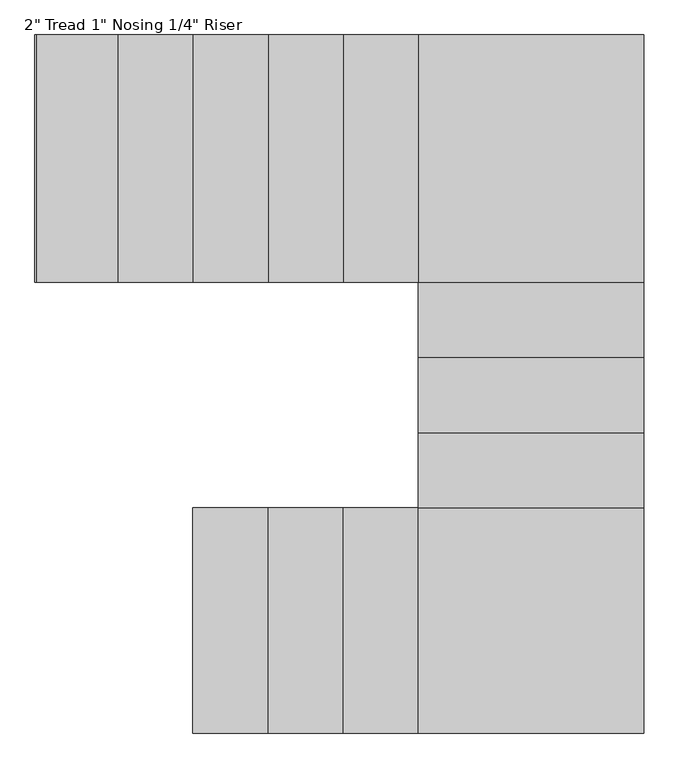
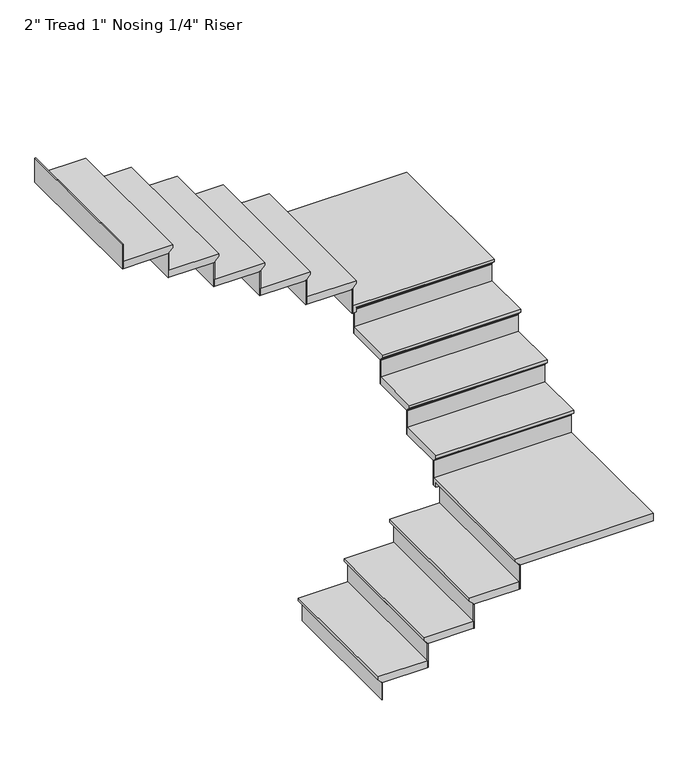
"""IFC4 building model written with IfcOpenShell, lengths in millimetres: stair flight geometry."""

from ifc_helpers import new_model, si_unit, origin, place, context, project, spatial, faceted_brep, source, transform, mapped, element, save


def stair_flight_68b2e5de(model_context):
    return source(origin(), model_context, "Body", "Brep", [
        faceted_brep([(938.5174794, -182.0870507, 16152.2833333), (938.5174794, -182.0870507, 16171.3333333), (938.5174794, 732.3129493, 16171.3333333), (938.5174794, 732.3129493, 16152.2833333), (963.9174794, -182.0870507, 16126.8833333), (963.9174794, 732.3129493, 16126.8833333), (1268.7174794, -182.0870507, 16171.3333333), (1268.7174794, 732.3129493, 16171.3333333), (963.9174794, 732.3129493, 16120.5333333), (1268.7174794, 732.3129493, 16120.5333333), (1268.7174794, -182.0870507, 16120.5333333), (963.9174794, -182.0870507, 16120.5333333)], [[[0, 1, 2, 3]], [[4, 0, 3, 5]], [[2, 1, 6, 7]], [[8, 9, 10, 11]], [[2, 7, 9, 8, 5, 3]], [[8, 11, 4, 5]], [[6, 1, 0, 4, 11, 10]], [[7, 6, 10, 9]]]),
        faceted_brep([(963.9174794, -182.0870507, 16120.5333333), (963.9174794, -182.0870507, 16002.0), (970.2674794, -182.0870507, 16002.0), (970.2674794, -182.0870507, 16120.5333333), (963.9174794, 732.3129493, 16120.5333333), (970.2674794, 732.3129493, 16120.5333333), (970.2674794, 732.3129493, 16002.0), (963.9174794, 732.3129493, 16002.0)], [[[0, 1, 2, 3]], [[4, 5, 6, 7]], [[1, 0, 4, 7]], [[2, 1, 7, 6]], [[3, 2, 6, 5]], [[0, 3, 5, 4]]]),
        faceted_brep([(1268.7174794, -182.0870507, 16289.8666667), (1268.7174794, -182.0870507, 16120.5333333), (1275.0674794, -182.0870507, 16120.5333333), (1275.0674794, -182.0870507, 16289.8666667), (1268.7174794, 732.3129493, 16289.8666667), (1275.0674794, 732.3129493, 16289.8666667), (1275.0674794, 732.3129493, 16120.5333333), (1268.7174794, 732.3129493, 16120.5333333)], [[[0, 1, 2, 3]], [[4, 5, 6, 7]], [[1, 0, 4, 7]], [[2, 1, 7, 6]], [[3, 2, 6, 5]], [[0, 3, 5, 4]]]),
        faceted_brep([(1243.3174794, 732.3129493, 16340.6666667), (1243.3174794, -182.0870507, 16340.6666667), (1573.5174794, -182.0870507, 16340.6666667), (1573.5174794, 732.3129493, 16340.6666667), (1268.7174794, 732.3129493, 16289.8666667), (1573.5174794, 732.3129493, 16289.8666667), (1573.5174794, -182.0870507, 16289.8666667), (1268.7174794, -182.0870507, 16289.8666667), (1268.7174794, 732.3129493, 16296.2166667), (1243.3174794, 732.3129493, 16321.6166667), (1268.7174794, -182.0870507, 16296.2166667), (1243.3174794, -182.0870507, 16321.6166667)], [[[0, 1, 2, 3]], [[4, 5, 6, 7]], [[0, 3, 5, 4, 8, 9]], [[4, 7, 10, 8]], [[2, 1, 11, 10, 7, 6]], [[3, 2, 6, 5]], [[11, 1, 0, 9]], [[10, 11, 9, 8]]]),
        faceted_brep([(1573.5174794, -182.0870507, 16459.2), (1573.5174794, -182.0870507, 16289.8666667), (1579.8674794, -182.0870507, 16289.8666667), (1579.8674794, -182.0870507, 16459.2), (1573.5174794, 732.3129493, 16459.2), (1579.8674794, 732.3129493, 16459.2), (1579.8674794, 732.3129493, 16289.8666667), (1573.5174794, 732.3129493, 16289.8666667)], [[[0, 1, 2, 3]], [[4, 5, 6, 7]], [[1, 0, 4, 7]], [[2, 1, 7, 6]], [[3, 2, 6, 5]], [[0, 3, 5, 4]]]),
        faceted_brep([(1548.1174794, 732.3129493, 16510.0), (1548.1174794, -182.0870507, 16510.0), (1878.3174794, -182.0870507, 16510.0), (1878.3174794, 732.3129493, 16510.0), (1573.5174794, 732.3129493, 16459.2), (1878.3174794, 732.3129493, 16459.2), (1878.3174794, -182.0870507, 16459.2), (1573.5174794, -182.0870507, 16459.2), (1573.5174794, 732.3129493, 16465.55), (1548.1174794, 732.3129493, 16490.95), (1573.5174794, -182.0870507, 16465.55), (1548.1174794, -182.0870507, 16490.95)], [[[0, 1, 2, 3]], [[4, 5, 6, 7]], [[0, 3, 5, 4, 8, 9]], [[4, 7, 10, 8]], [[2, 1, 11, 10, 7, 6]], [[3, 2, 6, 5]], [[11, 1, 0, 9]], [[10, 11, 9, 8]]]),
        faceted_brep([(1878.3174794, -182.0870507, 16628.5333333), (1878.3174794, -182.0870507, 16459.2), (1884.6674794, -182.0870507, 16459.2), (1884.6674794, -182.0870507, 16628.5333333), (1878.3174794, 732.3129493, 16628.5333333), (1884.6674794, 732.3129493, 16628.5333333), (1884.6674794, 732.3129493, 16459.2), (1878.3174794, 732.3129493, 16459.2)], [[[0, 1, 2, 3]], [[4, 5, 6, 7]], [[1, 0, 4, 7]], [[2, 1, 7, 6]], [[3, 2, 6, 5]], [[0, 3, 5, 4]]]),
        faceted_brep([(2767.3174794, -182.0870507, 16679.3333333), (2767.3174794, 757.7129493, 16679.3333333), (1852.9174794, 757.7129493, 16679.3333333), (1852.9174794, -182.0870507, 16679.3333333), (1852.9174794, 732.3129493, 16628.5333333), (1852.9174794, 757.7129493, 16628.5333333), (2767.3174794, 757.7129493, 16628.5333333), (2767.3174794, -182.0870507, 16628.5333333), (1878.3174794, -182.0870507, 16628.5333333), (1878.3174794, 732.3129493, 16628.5333333), (1852.9174794, 732.3129493, 16660.2833333), (1852.9174794, -182.0870507, 16660.2833333), (1878.3174794, 732.3129493, 16634.8833333), (1878.3174794, -182.0870507, 16634.8833333)], [[[0, 1, 2, 3]], [[4, 5, 6, 7, 8, 9]], [[3, 2, 5, 4, 10, 11]], [[4, 9, 12, 10]], [[9, 8, 13, 12]], [[0, 3, 11, 13, 8, 7]], [[1, 0, 7, 6]], [[2, 1, 6, 5]], [[13, 11, 10, 12]]]),
        faceted_brep([(2767.3174794, 757.7129493, 16797.8666667), (2767.3174794, 757.7129493, 16628.5333333), (2767.3174794, 764.0629493, 16628.5333333), (2767.3174794, 764.0629493, 16797.8666667), (1852.9174794, 757.7129493, 16797.8666667), (1852.9174794, 764.0629493, 16797.8666667), (1852.9174794, 764.0629493, 16628.5333333), (1852.9174794, 757.7129493, 16628.5333333)], [[[0, 1, 2, 3]], [[4, 5, 6, 7]], [[1, 0, 4, 7]], [[2, 1, 7, 6]], [[3, 2, 6, 5]], [[0, 3, 5, 4]]]),
        faceted_brep([(1852.9174794, 732.3129493, 16848.6666667), (2767.3174794, 732.3129493, 16848.6666667), (2767.3174794, 1062.5129493, 16848.6666667), (1852.9174794, 1062.5129493, 16848.6666667), (1852.9174794, 757.7129493, 16797.8666667), (1852.9174794, 1062.5129493, 16797.8666667), (2767.3174794, 1062.5129493, 16797.8666667), (2767.3174794, 757.7129493, 16797.8666667), (1852.9174794, 757.7129493, 16804.2166667), (1852.9174794, 732.3129493, 16829.6166667), (2767.3174794, 757.7129493, 16804.2166667), (2767.3174794, 732.3129493, 16829.6166667)], [[[0, 1, 2, 3]], [[4, 5, 6, 7]], [[0, 3, 5, 4, 8, 9]], [[4, 7, 10, 8]], [[2, 1, 11, 10, 7, 6]], [[3, 2, 6, 5]], [[11, 1, 0, 9]], [[10, 11, 9, 8]]]),
        faceted_brep([(2767.3174794, 1062.5129493, 16967.2), (2767.3174794, 1062.5129493, 16797.8666667), (2767.3174794, 1068.8629493, 16797.8666667), (2767.3174794, 1068.8629493, 16967.2), (1852.9174794, 1062.5129493, 16967.2), (1852.9174794, 1068.8629493, 16967.2), (1852.9174794, 1068.8629493, 16797.8666667), (1852.9174794, 1062.5129493, 16797.8666667)], [[[0, 1, 2, 3]], [[4, 5, 6, 7]], [[1, 0, 4, 7]], [[2, 1, 7, 6]], [[3, 2, 6, 5]], [[0, 3, 5, 4]]]),
        faceted_brep([(1852.9174794, 1037.1129493, 17018.0), (2767.3174794, 1037.1129493, 17018.0), (2767.3174794, 1367.3129493, 17018.0), (1852.9174794, 1367.3129493, 17018.0), (1852.9174794, 1062.5129493, 16967.2), (1852.9174794, 1367.3129493, 16967.2), (2767.3174794, 1367.3129493, 16967.2), (2767.3174794, 1062.5129493, 16967.2), (1852.9174794, 1062.5129493, 16973.55), (1852.9174794, 1037.1129493, 16998.95), (2767.3174794, 1062.5129493, 16973.55), (2767.3174794, 1037.1129493, 16998.95)], [[[0, 1, 2, 3]], [[4, 5, 6, 7]], [[0, 3, 5, 4, 8, 9]], [[4, 7, 10, 8]], [[2, 1, 11, 10, 7, 6]], [[3, 2, 6, 5]], [[11, 1, 0, 9]], [[10, 11, 9, 8]]]),
        faceted_brep([(2767.3174794, 1367.3129493, 17136.5333333), (2767.3174794, 1367.3129493, 16967.2), (2767.3174794, 1373.6629493, 16967.2), (2767.3174794, 1373.6629493, 17136.5333333), (1852.9174794, 1367.3129493, 17136.5333333), (1852.9174794, 1373.6629493, 17136.5333333), (1852.9174794, 1373.6629493, 16967.2), (1852.9174794, 1367.3129493, 16967.2)], [[[0, 1, 2, 3]], [[4, 5, 6, 7]], [[1, 0, 4, 7]], [[2, 1, 7, 6]], [[3, 2, 6, 5]], [[0, 3, 5, 4]]]),
        faceted_brep([(1852.9174794, 1341.9129493, 17187.3333333), (2767.3174794, 1341.9129493, 17187.3333333), (2767.3174794, 1672.1129493, 17187.3333333), (1852.9174794, 1672.1129493, 17187.3333333), (1852.9174794, 1367.3129493, 17136.5333333), (1852.9174794, 1672.1129493, 17136.5333333), (2767.3174794, 1672.1129493, 17136.5333333), (2767.3174794, 1367.3129493, 17136.5333333), (1852.9174794, 1367.3129493, 17142.8833333), (1852.9174794, 1341.9129493, 17168.2833333), (2767.3174794, 1367.3129493, 17142.8833333), (2767.3174794, 1341.9129493, 17168.2833333)], [[[0, 1, 2, 3]], [[4, 5, 6, 7]], [[0, 3, 5, 4, 8, 9]], [[4, 7, 10, 8]], [[2, 1, 11, 10, 7, 6]], [[3, 2, 6, 5]], [[11, 1, 0, 9]], [[10, 11, 9, 8]]]),
        faceted_brep([(2767.3174794, 1672.1129493, 17305.8666667), (2767.3174794, 1672.1129493, 17136.5333333), (2767.3174794, 1678.4629493, 17136.5333333), (2767.3174794, 1678.4629493, 17305.8666667), (1852.9174794, 1672.1129493, 17305.8666667), (1852.9174794, 1678.4629493, 17305.8666667), (1852.9174794, 1678.4629493, 17136.5333333), (1852.9174794, 1672.1129493, 17136.5333333)], [[[0, 1, 2, 3]], [[4, 5, 6, 7]], [[1, 0, 4, 7]], [[2, 1, 7, 6]], [[3, 2, 6, 5]], [[0, 3, 5, 4]]]),
        faceted_brep([(2767.3174794, 2650.0129493, 17356.6666667), (1827.5174794, 2650.0129493, 17356.6666667), (1827.5174794, 1646.7129493, 17356.6666667), (2767.3174794, 1646.7129493, 17356.6666667), (1852.9174794, 1646.7129493, 17305.8666667), (1827.5174794, 1646.7129493, 17305.8666667), (1827.5174794, 2650.0129493, 17305.8666667), (2767.3174794, 2650.0129493, 17305.8666667), (2767.3174794, 1672.1129493, 17305.8666667), (1852.9174794, 1672.1129493, 17305.8666667), (1852.9174794, 1646.7129493, 17337.6166667), (2767.3174794, 1646.7129493, 17337.6166667), (1852.9174794, 1672.1129493, 17312.2166667), (2767.3174794, 1672.1129493, 17312.2166667)], [[[0, 1, 2, 3]], [[4, 5, 6, 7, 8, 9]], [[3, 2, 5, 4, 10, 11]], [[4, 9, 12, 10]], [[9, 8, 13, 12]], [[0, 3, 11, 13, 8, 7]], [[1, 0, 7, 6]], [[2, 1, 6, 5]], [[13, 11, 10, 12]]]),
        faceted_brep([(1827.5174794, 2650.0129493, 17475.2), (1827.5174794, 2650.0129493, 17305.8666667), (1821.1674794, 2650.0129493, 17305.8666667), (1821.1674794, 2650.0129493, 17475.2), (1827.5174794, 1646.7129493, 17475.2), (1821.1674794, 1646.7129493, 17475.2), (1821.1674794, 1646.7129493, 17305.8666667), (1827.5174794, 1646.7129493, 17305.8666667)], [[[0, 1, 2, 3]], [[4, 5, 6, 7]], [[1, 0, 4, 7]], [[2, 1, 7, 6]], [[3, 2, 6, 5]], [[0, 3, 5, 4]]]),
        faceted_brep([(1852.9174794, 1646.7129493, 17526.0), (1852.9174794, 2650.0129493, 17526.0), (1522.7174794, 2650.0129493, 17526.0), (1522.7174794, 1646.7129493, 17526.0), (1827.5174794, 1646.7129493, 17475.2), (1522.7174794, 1646.7129493, 17475.2), (1522.7174794, 2650.0129493, 17475.2), (1827.5174794, 2650.0129493, 17475.2), (1827.5174794, 1646.7129493, 17481.55), (1852.9174794, 1646.7129493, 17506.95), (1827.5174794, 2650.0129493, 17481.55), (1852.9174794, 2650.0129493, 17506.95)], [[[0, 1, 2, 3]], [[4, 5, 6, 7]], [[0, 3, 5, 4, 8, 9]], [[4, 7, 10, 8]], [[2, 1, 11, 10, 7, 6]], [[3, 2, 6, 5]], [[11, 1, 0, 9]], [[10, 11, 9, 8]]]),
        faceted_brep([(1522.7174794, 2650.0129493, 17644.5333333), (1522.7174794, 2650.0129493, 17475.2), (1516.3674794, 2650.0129493, 17475.2), (1516.3674794, 2650.0129493, 17644.5333333), (1522.7174794, 1646.7129493, 17644.5333333), (1516.3674794, 1646.7129493, 17644.5333333), (1516.3674794, 1646.7129493, 17475.2), (1522.7174794, 1646.7129493, 17475.2)], [[[0, 1, 2, 3]], [[4, 5, 6, 7]], [[1, 0, 4, 7]], [[2, 1, 7, 6]], [[3, 2, 6, 5]], [[0, 3, 5, 4]]]),
        faceted_brep([(1548.1174794, 1646.7129493, 17695.3333333), (1548.1174794, 2650.0129493, 17695.3333333), (1217.9174794, 2650.0129493, 17695.3333333), (1217.9174794, 1646.7129493, 17695.3333333), (1522.7174794, 1646.7129493, 17644.5333333), (1217.9174794, 1646.7129493, 17644.5333333), (1217.9174794, 2650.0129493, 17644.5333333), (1522.7174794, 2650.0129493, 17644.5333333), (1522.7174794, 1646.7129493, 17650.8833333), (1548.1174794, 1646.7129493, 17676.2833333), (1522.7174794, 2650.0129493, 17650.8833333), (1548.1174794, 2650.0129493, 17676.2833333)], [[[0, 1, 2, 3]], [[4, 5, 6, 7]], [[0, 3, 5, 4, 8, 9]], [[4, 7, 10, 8]], [[2, 1, 11, 10, 7, 6]], [[3, 2, 6, 5]], [[11, 1, 0, 9]], [[10, 11, 9, 8]]]),
        faceted_brep([(1217.9174794, 2650.0129493, 17813.8666667), (1217.9174794, 2650.0129493, 17644.5333333), (1211.5674794, 2650.0129493, 17644.5333333), (1211.5674794, 2650.0129493, 17813.8666667), (1217.9174794, 1646.7129493, 17813.8666667), (1211.5674794, 1646.7129493, 17813.8666667), (1211.5674794, 1646.7129493, 17644.5333333), (1217.9174794, 1646.7129493, 17644.5333333)], [[[0, 1, 2, 3]], [[4, 5, 6, 7]], [[1, 0, 4, 7]], [[2, 1, 7, 6]], [[3, 2, 6, 5]], [[0, 3, 5, 4]]]),
        faceted_brep([(1243.3174794, 1646.7129493, 17864.6666667), (1243.3174794, 2650.0129493, 17864.6666667), (913.1174794, 2650.0129493, 17864.6666667), (913.1174794, 1646.7129493, 17864.6666667), (1217.9174794, 1646.7129493, 17813.8666667), (913.1174794, 1646.7129493, 17813.8666667), (913.1174794, 2650.0129493, 17813.8666667), (1217.9174794, 2650.0129493, 17813.8666667), (1217.9174794, 1646.7129493, 17820.2166667), (1243.3174794, 1646.7129493, 17845.6166667), (1217.9174794, 2650.0129493, 17820.2166667), (1243.3174794, 2650.0129493, 17845.6166667)], [[[0, 1, 2, 3]], [[4, 5, 6, 7]], [[0, 3, 5, 4, 8, 9]], [[4, 7, 10, 8]], [[2, 1, 11, 10, 7, 6]], [[3, 2, 6, 5]], [[11, 1, 0, 9]], [[10, 11, 9, 8]]]),
        faceted_brep([(913.1174794, 2650.0129493, 17983.2), (913.1174794, 2650.0129493, 17813.8666667), (906.7674794, 2650.0129493, 17813.8666667), (906.7674794, 2650.0129493, 17983.2), (913.1174794, 1646.7129493, 17983.2), (906.7674794, 1646.7129493, 17983.2), (906.7674794, 1646.7129493, 17813.8666667), (913.1174794, 1646.7129493, 17813.8666667)], [[[0, 1, 2, 3]], [[4, 5, 6, 7]], [[1, 0, 4, 7]], [[2, 1, 7, 6]], [[3, 2, 6, 5]], [[0, 3, 5, 4]]]),
        faceted_brep([(938.5174794, 1646.7129493, 18034.0), (938.5174794, 2650.0129493, 18034.0), (608.3174794, 2650.0129493, 18034.0), (608.3174794, 1646.7129493, 18034.0), (913.1174794, 1646.7129493, 17983.2), (608.3174794, 1646.7129493, 17983.2), (608.3174794, 2650.0129493, 17983.2), (913.1174794, 2650.0129493, 17983.2), (913.1174794, 1646.7129493, 17989.55), (938.5174794, 1646.7129493, 18014.95), (913.1174794, 2650.0129493, 17989.55), (938.5174794, 2650.0129493, 18014.95)], [[[0, 1, 2, 3]], [[4, 5, 6, 7]], [[0, 3, 5, 4, 8, 9]], [[4, 7, 10, 8]], [[2, 1, 11, 10, 7, 6]], [[3, 2, 6, 5]], [[11, 1, 0, 9]], [[10, 11, 9, 8]]]),
        faceted_brep([(608.3174794, 2650.0129493, 18152.5333333), (608.3174794, 2650.0129493, 17983.2), (601.9674794, 2650.0129493, 17983.2), (601.9674794, 2650.0129493, 18152.5333333), (608.3174794, 1646.7129493, 18152.5333333), (601.9674794, 1646.7129493, 18152.5333333), (601.9674794, 1646.7129493, 17983.2), (608.3174794, 1646.7129493, 17983.2)], [[[0, 1, 2, 3]], [[4, 5, 6, 7]], [[1, 0, 4, 7]], [[2, 1, 7, 6]], [[3, 2, 6, 5]], [[0, 3, 5, 4]]]),
        faceted_brep([(303.5174794, 2650.0129493, 18321.8666667), (303.5174794, 2650.0129493, 18152.5333333), (297.1674794, 2650.0129493, 18152.5333333), (297.1674794, 2650.0129493, 18321.8666667), (303.5174794, 1646.7129493, 18321.8666667), (297.1674794, 1646.7129493, 18321.8666667), (297.1674794, 1646.7129493, 18152.5333333), (303.5174794, 1646.7129493, 18152.5333333)], [[[0, 1, 2, 3]], [[4, 5, 6, 7]], [[1, 0, 4, 7]], [[2, 1, 7, 6]], [[3, 2, 6, 5]], [[0, 3, 5, 4]]]),
        faceted_brep([(633.7174794, 1646.7129493, 18203.3333333), (633.7174794, 2650.0129493, 18203.3333333), (303.5174794, 2650.0129493, 18203.3333333), (303.5174794, 1646.7129493, 18203.3333333), (608.3174794, 1646.7129493, 18152.5333333), (303.5174794, 1646.7129493, 18152.5333333), (303.5174794, 2650.0129493, 18152.5333333), (608.3174794, 2650.0129493, 18152.5333333), (608.3174794, 1646.7129493, 18158.8833333), (633.7174794, 1646.7129493, 18184.2833333), (608.3174794, 2650.0129493, 18158.8833333), (633.7174794, 2650.0129493, 18184.2833333)], [[[0, 1, 2, 3]], [[4, 5, 6, 7]], [[0, 3, 5, 4, 8, 9]], [[4, 7, 10, 8]], [[2, 1, 11, 10, 7, 6]], [[3, 2, 6, 5]], [[11, 1, 0, 9]], [[10, 11, 9, 8]]]),
    ])


if __name__ == "__main__":
    model = new_model("IFC4")
    model_context = context("Model", 3, world=origin())
    ifc_project = project(units=[si_unit("LENGTHUNIT", "METRE", prefix="MILLI")], contexts=[model_context])
    site = spatial("IfcSite", under=ifc_project)
    building = spatial("IfcBuilding", under=site)
    placement = place(None, origin())
    stair_flight_shape = stair_flight_68b2e5de(model_context)
    element("IfcStairFlight", 1, ObjectType="2\" Tread 1\" Nosing 1/4\" Riser", at=placement, inside=building, context=model_context, shape_type="MappedRepresentation", body=[
        mapped(stair_flight_shape, transform((0.0, 0.0, 0.0), x_axis=(1.0, 0.0, 0.0), y_axis=(0.0, 1.0, 0.0), z_axis=(0.0, 0.0, 1.0))),
    ])
    save(model, "model.ifc")
